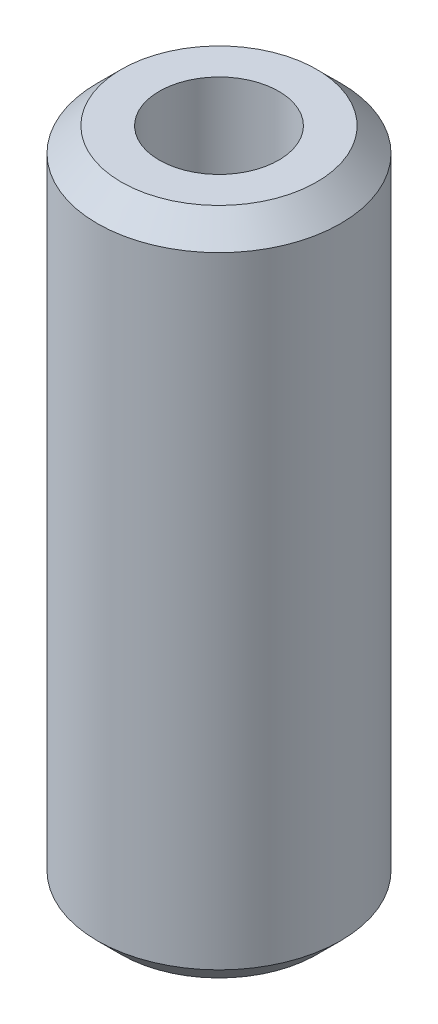
ISO-10303-21;
HEADER;
FILE_DESCRIPTION(('STEP AP214'),'2;1');
FILE_NAME('part.step','',(''),(''),'','','');
FILE_SCHEMA(('AUTOMOTIVE_DESIGN { 1 0 10303 214 1 1 1 1 }'));
ENDSEC;
DATA;
#1=APPLICATION_CONTEXT('core data for automotive mechanical design processes');
#2=APPLICATION_PROTOCOL_DEFINITION('international standard','automotive_design',2000,#1);
#3=PRODUCT_CONTEXT('',#1,'mechanical');
#4=PRODUCT('Part','Part','',(#3));
#5=PRODUCT_RELATED_PRODUCT_CATEGORY('part','',(#4));
#6=PRODUCT_DEFINITION_FORMATION('','',#4);
#7=PRODUCT_DEFINITION_CONTEXT('part definition',#1,'design');
#8=PRODUCT_DEFINITION('design','',#6,#7);
#9=PRODUCT_DEFINITION_SHAPE('','',#8);
#10=(LENGTH_UNIT() NAMED_UNIT(*) SI_UNIT(.MILLI.,.METRE.));
#11=(NAMED_UNIT(*) PLANE_ANGLE_UNIT() SI_UNIT($,.RADIAN.));
#12=(NAMED_UNIT(*) SI_UNIT($,.STERADIAN.) SOLID_ANGLE_UNIT());
#13=UNCERTAINTY_MEASURE_WITH_UNIT(LENGTH_MEASURE(1.E-05),#10,'distance_accuracy_value','');
#14=(GEOMETRIC_REPRESENTATION_CONTEXT(3) GLOBAL_UNCERTAINTY_ASSIGNED_CONTEXT((#13)) GLOBAL_UNIT_ASSIGNED_CONTEXT((#10,
#11,#12)) REPRESENTATION_CONTEXT('',''));
#15=CARTESIAN_POINT('',(0.,0.,0.));
#16=DIRECTION('',(0.,0.,1.));
#17=DIRECTION('',(1.,0.,0.));
#18=AXIS2_PLACEMENT_3D('',#15,#16,#17);
#19=CARTESIAN_POINT('',(0.,34.925,0.));
#20=DIRECTION('',(0.,1.,0.));
#21=DIRECTION('',(0.,0.,1.));
#22=AXIS2_PLACEMENT_3D('',#19,#20,#21);
#23=PLANE('',#22);
#24=CARTESIAN_POINT('',(0.,34.925,0.));
#25=DIRECTION('',(0.,1.,0.));
#26=DIRECTION('',(0.,0.,1.));
#27=AXIS2_PLACEMENT_3D('',#24,#25,#26);
#28=CIRCLE('',#27,10.2);
#29=CARTESIAN_POINT('',(0.,34.925,10.2));
#30=VERTEX_POINT('',#29);
#31=EDGE_CURVE('E10',#30,#30,#28,.T.);
#32=ORIENTED_EDGE('',*,*,#31,.T.);
#33=EDGE_LOOP('',(#32));
#34=FACE_BOUND('',#33,.T.);
#35=CARTESIAN_POINT('',(0.,34.925,0.));
#36=DIRECTION('',(0.,1.,0.));
#37=DIRECTION('',(0.,0.,1.));
#38=AXIS2_PLACEMENT_3D('',#35,#36,#37);
#39=CIRCLE('',#38,6.235);
#40=CARTESIAN_POINT('',(0.,34.925,6.235));
#41=VERTEX_POINT('',#40);
#42=EDGE_CURVE('E58',#41,#41,#39,.T.);
#43=ORIENTED_EDGE('',*,*,#42,.F.);
#44=EDGE_LOOP('',(#43));
#45=FACE_BOUND('',#44,.T.);
#46=ADVANCED_FACE('F39',(#34,#45),#23,.T.);
#47=CARTESIAN_POINT('',(0.,-34.925,0.));
#48=DIRECTION('',(0.,1.,0.));
#49=DIRECTION('',(0.,0.,1.));
#50=AXIS2_PLACEMENT_3D('',#47,#48,#49);
#51=PLANE('',#50);
#52=CARTESIAN_POINT('',(0.,-34.925,0.));
#53=DIRECTION('',(0.,1.,0.));
#54=DIRECTION('',(0.,0.,1.));
#55=AXIS2_PLACEMENT_3D('',#52,#53,#54);
#56=CIRCLE('',#55,10.2);
#57=CARTESIAN_POINT('',(0.,-34.925,10.2));
#58=VERTEX_POINT('',#57);
#59=EDGE_CURVE('E50',#58,#58,#56,.F.);
#60=ORIENTED_EDGE('',*,*,#59,.T.);
#61=EDGE_LOOP('',(#60));
#62=FACE_BOUND('',#61,.T.);
#63=CARTESIAN_POINT('',(0.,-34.925,0.));
#64=DIRECTION('',(0.,1.,0.));
#65=DIRECTION('',(0.,0.,1.));
#66=AXIS2_PLACEMENT_3D('',#63,#64,#65);
#67=CIRCLE('',#66,6.235);
#68=CARTESIAN_POINT('',(0.,-34.925,6.235));
#69=VERTEX_POINT('',#68);
#70=EDGE_CURVE('E64',#69,#69,#67,.T.);
#71=ORIENTED_EDGE('',*,*,#70,.T.);
#72=EDGE_LOOP('',(#71));
#73=FACE_BOUND('',#72,.T.);
#74=ADVANCED_FACE('F72',(#62,#73),#51,.F.);
#75=CARTESIAN_POINT('',(0.,34.925,0.));
#76=DIRECTION('',(0.,-1.,0.));
#77=DIRECTION('',(0.,0.,-1.));
#78=AXIS2_PLACEMENT_3D('',#75,#76,#77);
#79=CYLINDRICAL_SURFACE('',#78,12.7);
#80=CARTESIAN_POINT('',(0.,-32.425,0.));
#81=DIRECTION('',(0.,1.,0.));
#82=DIRECTION('',(0.,0.,1.));
#83=AXIS2_PLACEMENT_3D('',#80,#81,#82);
#84=CIRCLE('',#83,12.7);
#85=CARTESIAN_POINT('',(0.,-32.425,12.7));
#86=VERTEX_POINT('',#85);
#87=EDGE_CURVE('E51',#86,#86,#84,.T.);
#88=ORIENTED_EDGE('',*,*,#87,.T.);
#89=EDGE_LOOP('',(#88));
#90=FACE_BOUND('',#89,.T.);
#91=CARTESIAN_POINT('',(0.,32.425,0.));
#92=DIRECTION('',(0.,1.,0.));
#93=DIRECTION('',(0.,0.,1.));
#94=AXIS2_PLACEMENT_3D('',#91,#92,#93);
#95=CIRCLE('',#94,12.7);
#96=CARTESIAN_POINT('',(0.,32.425,12.7));
#97=VERTEX_POINT('',#96);
#98=EDGE_CURVE('E54',#97,#97,#95,.F.);
#99=ORIENTED_EDGE('',*,*,#98,.T.);
#100=EDGE_LOOP('',(#99));
#101=FACE_BOUND('',#100,.T.);
#102=ADVANCED_FACE('F76',(#90,#101),#79,.T.);
#103=CARTESIAN_POINT('',(0.,34.925,0.));
#104=DIRECTION('',(0.,-1.,0.));
#105=DIRECTION('',(0.,0.,-1.));
#106=AXIS2_PLACEMENT_3D('',#103,#104,#105);
#107=CYLINDRICAL_SURFACE('',#106,6.235);
#108=ORIENTED_EDGE('',*,*,#42,.T.);
#109=EDGE_LOOP('',(#108));
#110=FACE_BOUND('',#109,.T.);
#111=ORIENTED_EDGE('',*,*,#70,.F.);
#112=EDGE_LOOP('',(#111));
#113=FACE_BOUND('',#112,.T.);
#114=ADVANCED_FACE('F70',(#110,#113),#107,.F.);
#115=CARTESIAN_POINT('',(0.,-32.425,0.));
#116=DIRECTION('',(0.,1.,0.));
#117=DIRECTION('',(0.,0.,1.));
#118=AXIS2_PLACEMENT_3D('',#115,#116,#117);
#119=CONICAL_SURFACE('',#118,12.7,0.785398163397449);
#120=ORIENTED_EDGE('',*,*,#59,.F.);
#121=EDGE_LOOP('',(#120));
#122=FACE_BOUND('',#121,.T.);
#123=ORIENTED_EDGE('',*,*,#87,.F.);
#124=EDGE_LOOP('',(#123));
#125=FACE_BOUND('',#124,.T.);
#126=ADVANCED_FACE('F84',(#122,#125),#119,.T.);
#127=CARTESIAN_POINT('',(0.,34.925,0.));
#128=DIRECTION('',(0.,-1.,0.));
#129=DIRECTION('',(0.,0.,-1.));
#130=AXIS2_PLACEMENT_3D('',#127,#128,#129);
#131=CONICAL_SURFACE('',#130,10.2,0.785398163397446);
#132=ORIENTED_EDGE('',*,*,#98,.F.);
#133=EDGE_LOOP('',(#132));
#134=FACE_BOUND('',#133,.T.);
#135=ORIENTED_EDGE('',*,*,#31,.F.);
#136=EDGE_LOOP('',(#135));
#137=FACE_BOUND('',#136,.T.);
#138=ADVANCED_FACE('F45',(#134,#137),#131,.T.);
#139=CLOSED_SHELL('',(#46,#74,#102,#114,#126,#138));
#140=MANIFOLD_SOLID_BREP('B2',#139);
#141=ADVANCED_BREP_SHAPE_REPRESENTATION('',(#18,#140),#14);
#142=SHAPE_DEFINITION_REPRESENTATION(#9,#141);
ENDSEC;
END-ISO-10303-21;
